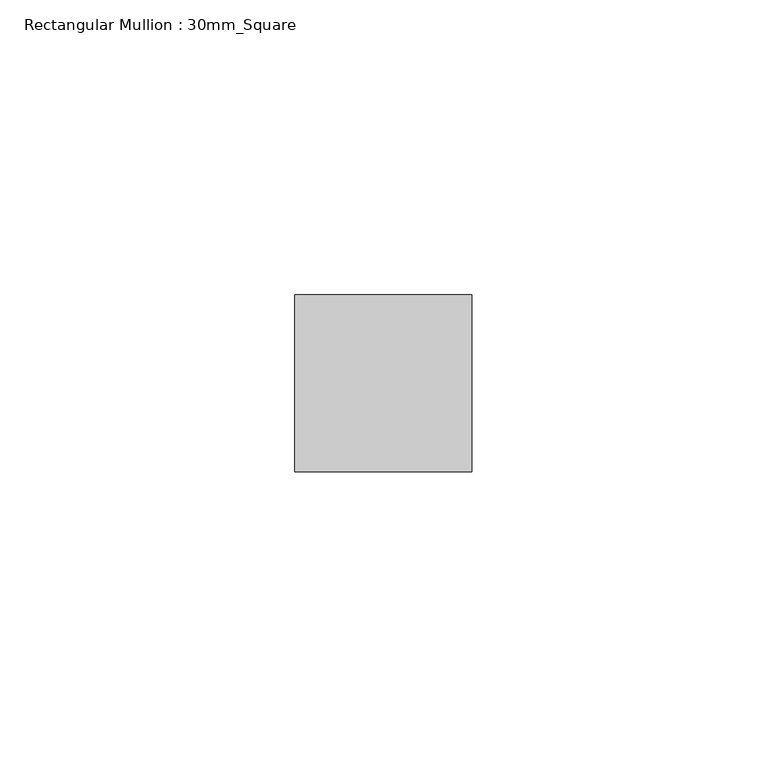
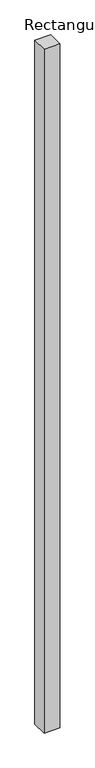
"""IFC4 building model written with IfcOpenShell, lengths in millimetres: member geometry, Rectangular Mullion : 30mm_Square."""

from ifc_helpers import new_model, si_unit, frame, origin, place, context, project, spatial, polyline, outline, extrude, source, transform, mapped, element, save


def rectangular_mullion_30mm_square_817e3251(model_context):
    return source(origin(), model_context, "Body", "SweptSolid", [
        extrude(outline(polyline([(0.0, 15.0), (0.0, -15.0), (-30.0, -15.0), (-30.0, 15.0), (0.0, 15.0)])), frame((0.0, 0.0, -1372.4911453), z_axis=(0.0, 0.0, 1.0), x_axis=(1.0, 0.0, 0.0)), (0.0, 0.0, 1.0), 1372.4911453),
    ])


if __name__ == "__main__":
    model = new_model("IFC4")
    model_context = context("Model", 3, world=origin())
    ifc_project = project(units=[si_unit("LENGTHUNIT", "METRE", prefix="MILLI")], contexts=[model_context])
    site = spatial("IfcSite", under=ifc_project)
    building = spatial("IfcBuilding", under=site)
    placement = place(None, origin())
    rectangular_mullion_30mm_square_shape = rectangular_mullion_30mm_square_817e3251(model_context)
    element("IfcMember", 1, ObjectType="Rectangular Mullion : 30mm_Square", at=placement, inside=building, context=model_context, shape_type="MappedRepresentation", body=[
        mapped(rectangular_mullion_30mm_square_shape, transform((0.0, 0.0, 0.0), x_axis=(1.0, 0.0, 0.0), y_axis=(0.0, 1.0, 0.0), z_axis=(0.0, 0.0, 1.0))),
    ])
    save(model, "model.ifc")

# Revit data of these elements
# Type "Rectangular Mullion : 30mm_Square"
#   Keynote = "H11"
#   built-in parameter 1007304 = 0.0984252 (stored number, unit not read)
#   built-in parameter 1007301 = 0.0492126 (stored number, unit not read)
#   built-in parameter 1007300 = 0.0492126 (stored number, unit not read)
# Element 1 (IfcMember, "Rectangular Mullion : 30mm_Square")
#   Materials on its faces: "Aluminium"
# Materials
#   "Aluminium": class "Metal", colour RGB 247 247 247, transparency 0, Description = "Aluminium 6061", Cost = 0
